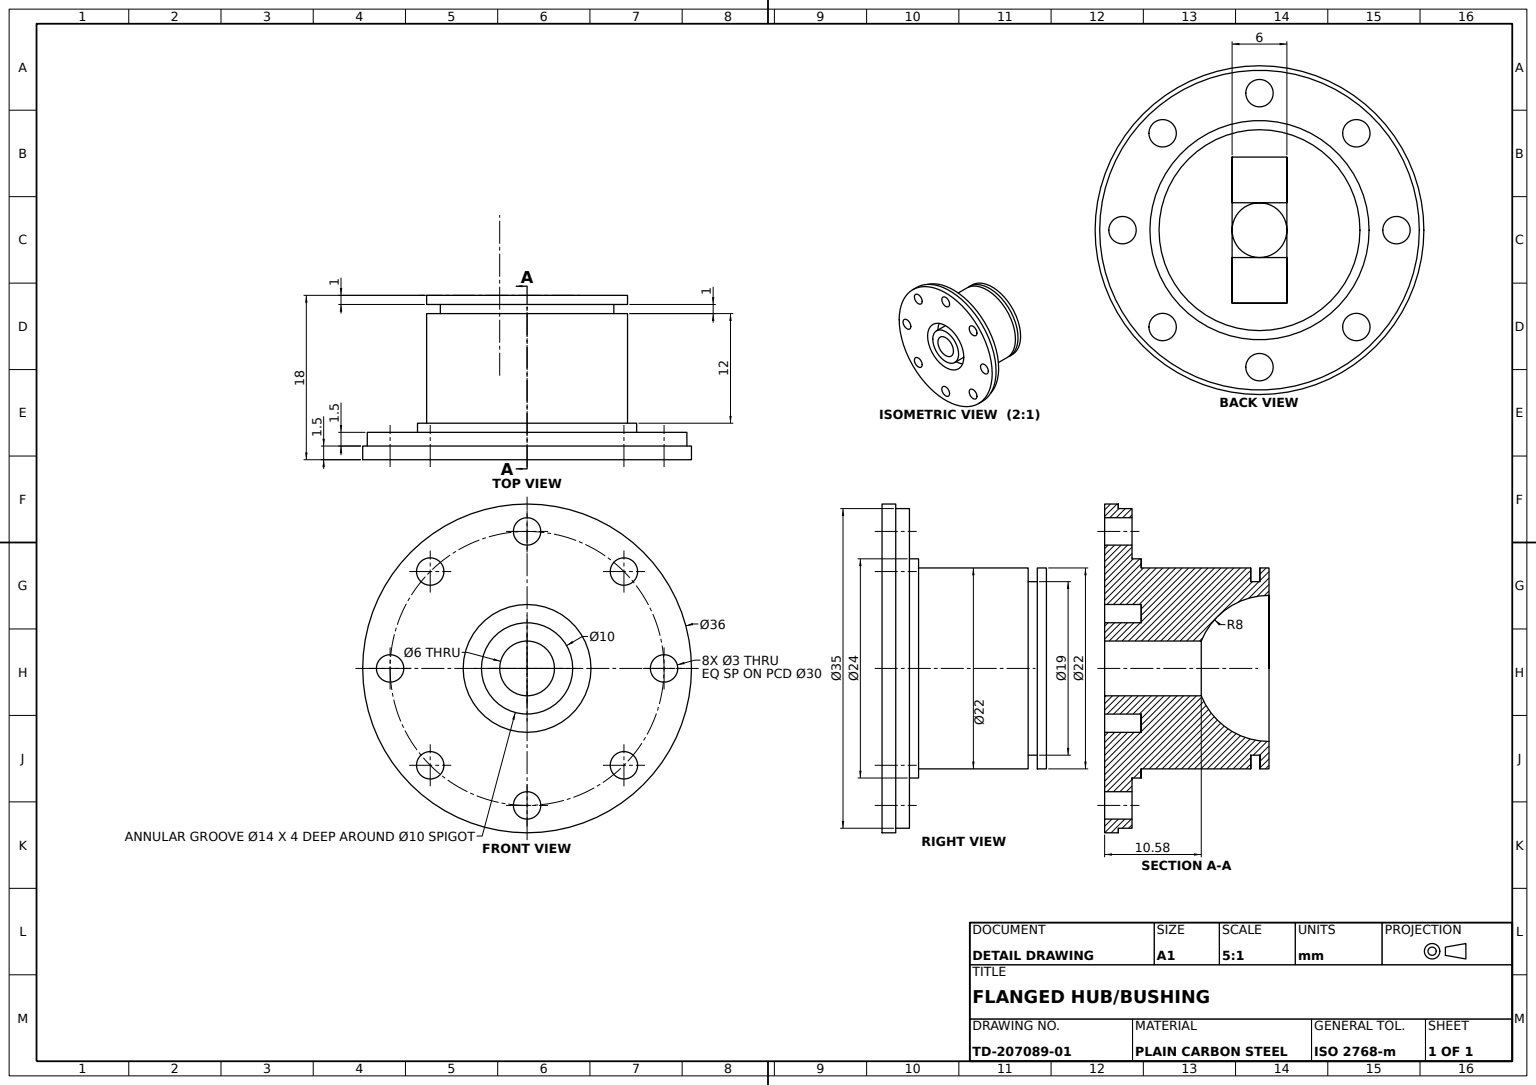
from build123d import *

# Parameters (mm, degrees)
BASE_LIP_SKETCH_22_R       = 11
BASE_LIP_22_DEPTH          = 1
GROOVE_SKETCH_19_R         = 9.5
GROOVE_NECK_19_DEPTH       = 1
SHANK_SKETCH_22_R          = 11
SHANK_22_DEPTH             = 12
COLLAR_SKETCH_24_R         = 12
COLLAR_24_DEPTH            = 1
FLANGE_LOWER_SKETCH_35_R   = 17.5
FLANGE_LOWER_STEP_35_DEPTH = 1.5
FLANGE_SKETCH_36_R         = 18
FLANGE_36_DEPTH            = 1.5
SIDE_WINDOW_CUT_DEPTH      = 3
BOLT_HOLES_SKETCH_8X_3_R   = 1.5
BOLT_HOLES_8X_3_DEPTH      = 6
RECESS_SKETCH_14_R         = 7
RECESS_14_DEPTH            = 4
INNER_SPIGOT_SKETCH_10_R   = 5
INNER_SPIGOT_10_DEPTH      = 4
BORE_SKETCH_6_R            = 3
THROUGH_BORE_6_DEPTH       = 10.58


with BuildPart() as part:
    # Base Lip Sketch Ø22 → Base Lip Ø22 (new body)
    with BuildSketch(Plane(origin=(0, 0, 0), x_dir=(1, 0, 0), z_dir=(0, 1, 0))):
        with Locations(Location((0, 0, 0), (0, 0, 270))):
            Circle(BASE_LIP_SKETCH_22_R)
    extrude(amount=BASE_LIP_22_DEPTH)

    # Groove Sketch Ø19 → Groove Neck Ø19 (add)
    with BuildSketch(Plane(origin=(0, 1, 0), x_dir=(1, 0, 0), z_dir=(0, 1, 0))):
        with Locations(Location((0, 0, 0), (0, 0, 270))):
            Circle(GROOVE_SKETCH_19_R)
    extrude(amount=GROOVE_NECK_19_DEPTH)

    # Shank Sketch Ø22 → Shank Ø22 (add)
    with BuildSketch(Plane(origin=(0, 2, 0), x_dir=(1, 0, 0), z_dir=(0, 1, 0))):
        with Locations(Location((0, 0, 0), (0, 0, 270))):
            Circle(SHANK_SKETCH_22_R)
    extrude(amount=SHANK_22_DEPTH)

    # Collar Sketch Ø24 → Collar Ø24 (add)
    with BuildSketch(Plane(origin=(0, 14, 0), x_dir=(1, 0, 0), z_dir=(0, 1, 0))):
        with Locations(Location((0, 0, 0), (0, 0, 270))):
            Circle(COLLAR_SKETCH_24_R)
    extrude(amount=COLLAR_24_DEPTH)

    # Flange Lower Sketch Ø35 → Flange Lower Step Ø35 (add)
    with BuildSketch(Plane(origin=(0, 15, 0), x_dir=(1, 0, 0), z_dir=(0, 1, 0))):
        with Locations(Location((0, 0, 0), (0, 0, 270))):
            Circle(FLANGE_LOWER_SKETCH_35_R)
    extrude(amount=FLANGE_LOWER_STEP_35_DEPTH)

    # Flange Sketch Ø36 → Flange Ø36 (add)
    with BuildSketch(Plane(origin=(0, 16.5, 0), x_dir=(1, 0, 0), z_dir=(0, 1, 0))):
        with Locations(Location((0, 0, 0), (0, 0, 270))):
            Circle(FLANGE_SKETCH_36_R)
    extrude(amount=FLANGE_36_DEPTH)

    # Side Window Sketch → Side Window Cut (cut, symmetric)
    with BuildSketch(Plane.XY):
        with BuildLine():
            Line((-8, 0), (8, 0))
            ThreePointArc((8, 0), (6.634312477, 4.474361508), (3, 7.42))
            Line((3, 7.42), (-3, 7.42))
            ThreePointArc((-3, 7.42), (-6.634312477, 4.474361508), (-8, 0))
        make_face()
    extrude(amount=SIDE_WINDOW_CUT_DEPTH, both=True, mode=Mode.SUBTRACT)

    # Bolt Holes Sketch 8xØ3 → Bolt Holes 8xØ3 (cut)
    with BuildSketch(Plane(origin=(0, 18, 0), x_dir=(1, 0, 0), z_dir=(0, 1, 0))):
        with Locations(Location((0, 15, 0), (0, 0, 270))):
            Circle(BOLT_HOLES_SKETCH_8X_3_R)
        with Locations(Location((10.606601718, 10.606601718, 0), (0, 0, 270))):
            Circle(BOLT_HOLES_SKETCH_8X_3_R)
        with Locations(Location((15, 0, 0), (0, 0, 270))):
            Circle(BOLT_HOLES_SKETCH_8X_3_R)
        with Locations(Location((10.606601718, -10.606601718, 0), (0, 0, 270))):
            Circle(BOLT_HOLES_SKETCH_8X_3_R)
        with Locations(Location((0, -15, 0), (0, 0, 270))):
            Circle(BOLT_HOLES_SKETCH_8X_3_R)
        with Locations(Location((-10.606601718, -10.606601718, 0), (0, 0, 270))):
            Circle(BOLT_HOLES_SKETCH_8X_3_R)
        with Locations(Location((-15, 0, 0), (0, 0, 270))):
            Circle(BOLT_HOLES_SKETCH_8X_3_R)
        with Locations(Location((-10.606601718, 10.606601718, 0), (0, 0, 270))):
            Circle(BOLT_HOLES_SKETCH_8X_3_R)
    extrude(amount=-BOLT_HOLES_8X_3_DEPTH, mode=Mode.SUBTRACT)

    # Recess Sketch Ø14 → Recess Ø14 (cut)
    with BuildSketch(Plane(origin=(0, 18, 0), x_dir=(1, 0, 0), z_dir=(0, 1, 0))):
        with Locations(Location((0, 0, 0), (0, 0, 270))):
            Circle(RECESS_SKETCH_14_R)
    extrude(amount=-RECESS_14_DEPTH, mode=Mode.SUBTRACT)

    # Inner Spigot Sketch Ø10 → Inner Spigot Ø10 (add)
    with BuildSketch(Plane(origin=(0, 18, 0), x_dir=(1, 0, 0), z_dir=(0, 1, 0))):
        with Locations(Location((0, 0, 0), (0, 0, 270))):
            Circle(INNER_SPIGOT_SKETCH_10_R)
    extrude(amount=-INNER_SPIGOT_10_DEPTH)

    # Bore Sketch Ø6 → Through Bore Ø6 (cut)
    with BuildSketch(Plane(origin=(0, 18, 0), x_dir=(1, 0, 0), z_dir=(0, 1, 0))):
        with Locations(Location((0, 0, 0), (0, 0, 270))):
            Circle(BORE_SKETCH_6_R)
    extrude(amount=-THROUGH_BORE_6_DEPTH, mode=Mode.SUBTRACT)


solid = part.part
